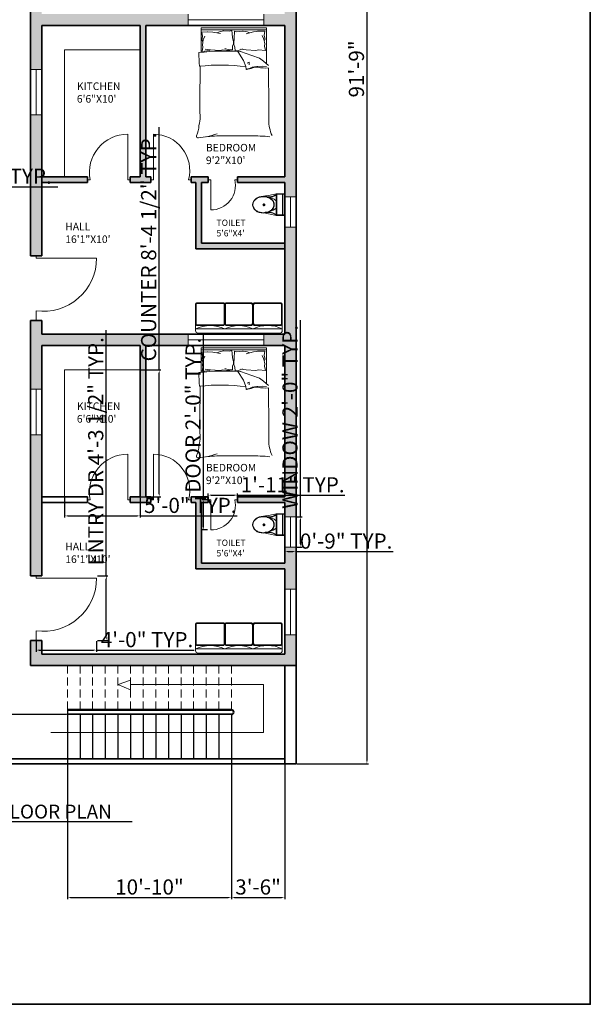
# Model space of a CAD drawing. Units: inches. Extents: x 1266 to 2869, y -408 to 3241.
# Tile 7 of 11: x 2416 to 2869, y 987 to 1767. Entities that reach past the tile are written whole.
import ezdxf

# ---------------------------------------------------------------- set-up
doc = ezdxf.new("R2010")
doc.units = ezdxf.units.IN
doc.linetypes.add('DASHED2', pattern=[9.525, 6.35, -3.175])
for name, color, linetype, lineweight in [('A-ANNO-DIMS', 2, 'Continuous', 18), ('A-ANNO-SYMB', 7, 'Continuous', 18), ('A-ANNO-TITL', 7, 'Continuous', 25), ('A-ANNO-TTLB', 7, 'Continuous', 35), ('A-AREA-IDEN', 7, 'Continuous', 18), ('A-DOOR', 4, 'Continuous', 18), ('A-FLOR-CASE', 9, 'Continuous', 18), ('A-FLOR-FIXT', 9, 'Continuous', 18), ('A-FLOR-STRS', 7, 'Continuous', 25), ('A-FLOR-STRS-OVHD', 8, 'DASHED2', 18), ('A-FURN', 8, 'Continuous', 18), ('A-GLAZ', 4, 'Continuous', 18), ('A-WALL', 7, 'Continuous', 35), ('A-WALL-PATT', 251, 'Continuous', 13)]:
    doc.layers.add(name, color=color, linetype=linetype, lineweight=lineweight)
doc.styles.get("Standard").update_dxf_attribs({"font": 'arial.ttf'})
doc.dimstyles.new('ISO-25', dxfattribs={"dimtxt": 12, "dimasz": 2.5, "dimexe": 1.25, "dimexo": 0.625, "dimtad": 1, "dimdec": 0, "dimlunit": 3, "dimtxsty": 'Standard', "dimcen": 2.5, "dimadec": 0, "dimazin": 0, "dimtfac": 1, "dimtdec": 0, "dimtmove": 0, "dimatfit": 3, "dimfxl": 1, "dimarcsym": 0})

# ---------------------------------------------------------------- blocks, each defined once
blk = doc.blocks.new('A$C31115884')
for p, q in [((283, 498), (223, 498)), ((258, 466), (258, 523)), ((0, 200), (0, 0)), ((520, 200), (0, 200)), ((510, 54), (0, 54)), ((10, 190), (10, 10)), ((510, 190), (10, 190)), ((10, 10), (510, 10)), ((510, 10), (510, 190)), ((520, 0), (520, 200)), ((0, 0), (520, 0))]:
    blk.add_line(p, q)
blk.add_circle((256, 496), 23.6)
for centre, radius, start, end in [((2778, -205), 2807, 165.4549, 171.7133), ((3237, 905), 2807, 188.2867, 194.5451), ((-295, 403), 365, 324.2091, 9.3499), ((-295, 403), 375, 324.2091, 9.3499), ((384, 406), 293, 190.2774, 224.1564), ((139, 406), 293, 315.8436, 2.6563), ((806, 403), 375, 179.2036, 215.7909), ((806, 403), 365, 170.6501, 215.7909)]:
    blk.add_arc(centre, radius, start, end)
blk.add_ellipse((256, 510), major_axis=(0, -261), ratio=0.772727)
blk.add_open_spline([(256, 259), (263, 259), (270, 260), (288, 262), (299, 265), (320, 273), (330, 278), (350, 291), (360, 299), (378, 316), (386, 326), (402, 347), (409, 358), (421, 383), (427, 395), (436, 422), (440, 436), (445, 465), (447, 480), (448, 509), (448, 524), (445, 553), (443, 568), (436, 596), (432, 610), (422, 636), (416, 649), (402, 672), (395, 683), (379, 703), (370, 712), (351, 728), (341, 735), (321, 746), (310, 751), (289, 757), (278, 759), (256, 761), (245, 761), (223, 757), (212, 754), (191, 746), (181, 741), (161, 728), (151, 720), (133, 703), (125, 693), (110, 672), (103, 660), (90, 636), (85, 623), (76, 596), (72, 582), (67, 553), (66, 538), (64, 509), (65, 494), (68, 465), (70, 450), (77, 422), (81, 408), (91, 382), (97, 370), (111, 346), (118, 335), (135, 316), (144, 307), (162, 291), (172, 284), (193, 273), (203, 269), (225, 262), (236, 260), (250, 259), (253, 259), (256, 259)], degree=3, knots=[0, 0, 0, 0, 0.110105, 0.110105, 0.285049, 0.285049, 0.459994, 0.459994, 0.634938, 0.634938, 0.809882, 0.809882, 0.984827, 0.984827, 1.159771, 1.159771, 1.334715, 1.334715, 1.50966, 1.50966, 1.684604, 1.684604, 1.859549, 1.859549, 2.034493, 2.034493, 2.209437, 2.209437, 2.384382, 2.384382, 2.559326, 2.559326, 2.73427, 2.73427, 2.909215, 2.909215, 3.084159, 3.084159, 3.259103, 3.259103, 3.434048, 3.434048, 3.608992, 3.608992, 3.783936, 3.783936, 3.958881, 3.958881, 4.133825, 4.133825, 4.30877, 4.30877, 4.483714, 4.483714, 4.658658, 4.658658, 4.833603, 4.833603, 5.008547, 5.008547, 5.183491, 5.183491, 5.358436, 5.358436, 5.53338, 5.53338, 5.708324, 5.708324, 5.883269, 5.883269, 6.058213, 6.058213, 6.233158, 6.233158, 6.283185, 6.283185, 6.283185, 6.283185])
blk = doc.blocks.new('*D5')
at = {"layer": 'A-ANNO-DIMS', "color": 0, "lineweight": -2, "transparency": 16777216}
for p, q in [((2636.08, 2278.35), (2692.86, 2278.35)), ((2691.61, 2275.85), (2691.61, 1179.85)), ((2636.08, 1177.35), (2692.86, 1177.35))]:
    blk.add_line(p, q, dxfattribs=at)
at = {"layer": 'A-ANNO-DIMS', "color": 0, "transparency": 16777216}
for points in [[(2691.19, 2275.85), (2692.02, 2275.85), (2691.61, 2278.35)], [(2691.19, 1179.85), (2692.02, 1179.85), (2691.61, 1177.35)]]:
    blk.add_solid(points, dxfattribs=at)
at = {"layer": 'Defpoints', "color": 0, "transparency": 16777216}
for p in [(2635.45, 2278.35), (2635.45, 1177.35), (2691.61, 1177.35)]:
    blk.add_point(p, dxfattribs=at)
at = {"layer": 'A-ANNO-DIMS', "color": 0, "transparency": 16777216, "insert": (2684.86, 1727.85), "char_height": 12, "attachment_point": 5, "rotation": 90}
blk.add_mtext('91\'-9"', dxfattribs=at)
blk = doc.blocks.new('BED-DOUBLE-2')
for p, q in [((3.76, 67.77), (3.76, 87.35)), ((3.76, 87.35), (55.42, 87.35)), ((55.42, 87.35), (55.42, 58.59)), ((3.76, 85.69), (55.42, 85.69)), ((4.21, 83.74), (8.84, 84.1)), ((4.21, 83.77), (4.84, 80.33)), ((4.84, 80.33), (4.37, 77.51)), ((5.46, 77.67), (6.55, 80.64)), ((8.84, 84.1), (8.96, 84.08)), ((8.96, 84.08), (13.09, 83.77)), ((13.09, 83.77), (19.03, 82.67)), ((16.06, 83.3), (18.25, 84.08)), ((18.25, 84.08), (21.37, 84.86)), ((21.37, 84.86), (21.72, 84.86)), ((21.72, 84.86), (26.53, 84.7)), ((26.53, 84.7), (28.09, 85.33)), ((28.09, 85.33), (28.71, 79.55)), ((28.71, 79.55), (29.34, 76.11)), ((29.98, 78.85), (29.57, 75.38)), ((30.24, 84.66), (29.98, 78.85)), ((31.84, 84.13), (30.24, 84.66)), ((36.63, 84.59), (31.84, 84.13)), ((36.98, 84.61), (36.63, 84.59)), ((40.14, 84.02), (36.98, 84.61)), ((45.31, 84.03), (39.45, 82.57)), ((42.38, 83.38), (40.14, 84.02)), ((49.42, 84.6), (45.31, 84.03)), ((54.17, 84.59), (48.33, 84.69)), ((48.33, 84.69), (49.42, 84.6)), ((53.31, 78.43), (52.03, 81.32)), ((54.17, 74.56), (53.31, 78.43)), ((54.17, 84.59), (53.76, 81.12)), ((53.76, 81.12), (54.41, 78.34)), ((54.41, 78.34), (53.85, 77.21)), ((4.37, 77.51), (4.99, 76.42)), ((4.52, 68.61), (5.15, 72.04)), ((4.84, 73.76), (5.46, 77.67)), ((5.15, 72.04), (4.84, 73.76)), ((6.9, 70.46), (11.26, 69.74)), ((26.06, 69.77), (22.66, 70.95)), ((29.34, 74.7), (28.71, 72.67)), ((28.71, 72.67), (28.71, 69.77)), ((29.34, 76.11), (29.34, 74.7)), ((29.57, 75.38), (29.66, 73.97)), ((29.66, 73.97), (30.41, 71.98)), ((30.41, 71.98), (30.59, 69.09)), ((33.24, 69.26), (36.56, 70.64)), ((35.2, 70.46), (39.56, 69.74)), ((53.97, 72.83), (54.17, 74.56)), ((54.81, 69.44), (53.97, 72.83)), ((10.03, 69.39), (4.52, 68.61)), ((11.26, 69.74), (10.03, 69.39)), ((11.26, 69.74), (18.84, 69.27)), ((18.84, 69.27), (20.95, 69.87)), ((20.95, 69.87), (26.5, 69.44)), ((28.71, 69.77), (26.06, 69.77)), ((30.59, 69.09), (33.24, 69.26)), ((32.71, 68.56), (37.24, 61.54)), ((43.94, 65.39), (34.92, 68.56)), ((39.56, 69.74), (47.14, 69.27)), ((49.96, 63.21), (43.94, 65.39)), ((47.14, 69.27), (49.26, 69.87)), ((49.26, 69.87), (54.81, 69.44)), ((53.15, 60.87), (49.96, 63.21)), ((37.24, 61.54), (39.08, 56.69)), ((39.08, 56.69), (39.42, 54.51)), ((39.42, 54.51), (42.1, 55.18)), ((40.12, 59.32), (41.78, 59.99)), ((41.87, 58.1), (41.78, 59.99, 4.18)), ((42.1, 55.18), (44.27, 56.19)), ((44.27, 56.19), (47.96, 56.69)), ((47.96, 56.69), (52.14, 57.02)), ((52.14, 57.02), (55.49, 56.69)), ((57.15, 57.36), (53.15, 60.87)), ((16.28, 1.69), (42.89, 1.69))]:
    blk.add_line(p, q)
for centre, radius, start, end in [((92.06, 65.63), 90.06, 178.72178, 185.60397), ((23.09, -109.45), 178.34, 86.08655, 96.78213), ((19.19, -81.63), 139.47, 81.78449, 96.90062), ((-180.86, 53.65), 183.89, 358.4762, 1.00819), ((33.68, 85.75), 32.06, 280.66171, 289.88058), ((47.29, 49.44), 6.73, 78.6608, 113.73842), ((55.49, 94.55), 39.11, 259.87628, 272.56571), ((197.03, 48.09), 139.99, 176.97912, 183.83645), ((524.11, 32.64), 521.39, 178.22771, 181.71854), ((39.61, 54.45), 0.199, 160.24637, 271.13765), ((-4874.07, 14.03), 4931.49, 0.00217, 0.28689), ((-29.08, 17.61), 32.04, 346.06484, 358.91125), ((-23.41, 11.38), 25.47, 337.97508, 356.652), ((82.33, 13.12), 24.93, 177.47136, 206.46809), ((1.18, 1.17), 1.18, 146.17358, 293.47814), ((23.16, -129.76), 131.62, 92.99578, 99.40907), ((-18.62, 112.98), 115.08, 283.38322, 287.70533), ((44.49, -142.12), 143.82, 84.4998, 90.63509)]:
    blk.add_arc(centre, radius, start, end)
blk = doc.blocks.new('DOOR-KITCHEN-R')
for p, q in [((31.78, 0), (31.78, 36)), ((0, 0), (2, 0)), ((33.78, 0), (31.78, 0))]:
    blk.add_line(p, q)
blk.add_arc((31.78, 5.68), 30.32, 90, 190.7956)
blk = doc.blocks.new('DOOR-BEDROOM-R')
for p, q in [((2, 0), (2, 36)), ((0, 0), (2, 0)), ((31.84, 0), (29.84, 0))]:
    blk.add_line(p, q)
blk.add_arc((2, 7.24), 28.76, 345.43182, 90)
blk = doc.blocks.new('DOOR-BATH-R')
for p, q in [((0, 24), (2, 24)), ((2, 24), (2, 0)), ((23.14, 24), (21.14, 24))]:
    blk.add_line(p, q)
blk.add_arc((2, 19.63), 19.63, 270, 12.84994)
blk = doc.blocks.new('DOOR-ENTRY-R')
for p, q in [((0, 51.27), (0, 49.27)), ((0, 49.27), (36, 49.27)), ((36, 49.27), (48, 49.27)), ((0, 5.68), (0, 7.68)), ((0, 0), (0, 5.68))]:
    blk.add_line(p, q)
blk.add_arc((5.98, 49.27), 42.02, 261.81164, 0)
blk = doc.blocks.new('WIN-PLAN-60')
for p, q in [((0, 9), (0, 0)), ((60, 4.5), (60, 9)), ((60, 9), (60, 0)), ((0, 4.5), (60, 4.5)), ((0, 0), (0, 4.5))]:
    blk.add_line(p, q)
blk = doc.blocks.new('WIN-PLAN-36')
for p, q in [((0, 36), (9, 36)), ((4.5, 36), (4.5, 0)), ((9, 36), (4.5, 36)), ((4.5, 0), (0, 0)), ((0, 0), (9, 0))]:
    blk.add_line(p, q)
blk = doc.blocks.new('WIN-PLAN-24')
for p, q in [((0, 24), (9, 24)), ((4.5, 24), (4.5, 0)), ((9, 24), (4.5, 24)), ((0, 0), (9, 0))]:
    blk.add_line(p, q)
blk = doc.blocks.new('COUNTER-KITCHEN')
for p, q in [((0, 0), (0, 100.54)), ((0, 100.54), (59.82, 100.54))]:
    blk.add_line(p, q)
blk = doc.blocks.new('STAIR-PATH-RETURN')
for p, q in [((63.2, 41.3), (53.5, 38.03)), ((63.2, 33.87), (63.2, 41.3)), ((53.2, 38.03), (63.2, 33.87)), ((53.5, 38.03), (53.2, 38.03)), ((168.66, 38.03), (63.2, 38.03)), ((168.66, 0), (168.66, 38.03)), ((0, 0), (168.66, 0))]:
    blk.add_line(p, q)
blk = doc.blocks.new('*D43')
at = {"layer": 'A-ANNO-DIMS', "color": 0, "lineweight": -2, "transparency": 16777216}
for p, q in [((2197.56, 1639.47), (2197.56, 1633.21)), ((2235.18, 1639.47), (2235.18, 1633.21)), ((2200.06, 1634.46), (2232.68, 1634.46)), ((2235.18, 1634.46), (2446.61, 1634.46))]:
    blk.add_line(p, q, dxfattribs=at)
at = {"layer": 'A-ANNO-DIMS', "color": 0, "transparency": 16777216}
for points in [[(2200.06, 1634.87), (2200.06, 1634.04), (2197.56, 1634.46)], [(2232.68, 1634.87), (2232.68, 1634.04), (2235.18, 1634.46)]]:
    blk.add_solid(points, dxfattribs=at)
at = {"layer": 'Defpoints', "color": 0, "transparency": 16777216}
for p in [(2197.56, 1640.1), (2235.18, 1640.1), (2235.18, 1634.46)]:
    blk.add_point(p, dxfattribs=at)
at = {"layer": 'A-ANNO-DIMS', "color": 0, "transparency": 16777216, "insert": (2342.14, 1641.29), "char_height": 12, "attachment_point": 5}
blk.add_mtext('KITCHEN DR 3\'-1 1/2" TYP.', dxfattribs=at)
blk = doc.blocks.new('*D49')
at = {"layer": 'A-ANNO-DIMS', "color": 0, "lineweight": -2, "transparency": 16777216}
for p, q in [((2527.03, 1489.38), (2527.03, 1681.65)), ((2512.58, 1489.38), (2528.28, 1489.38)), ((2527.03, 1391.35), (2527.03, 1486.88)), ((2512.58, 1388.85), (2528.28, 1388.85))]:
    blk.add_line(p, q, dxfattribs=at)
at = {"layer": 'A-ANNO-DIMS', "color": 0, "transparency": 16777216}
for points in [[(2526.61, 1486.88), (2527.45, 1486.88), (2527.03, 1489.38)], [(2526.61, 1391.35), (2527.45, 1391.35), (2527.03, 1388.85)]]:
    blk.add_solid(points, dxfattribs=at)
at = {"layer": 'Defpoints', "color": 0, "transparency": 16777216}
for p in [(2511.95, 1489.38), (2527.03, 1489.38), (2511.95, 1388.85)]:
    blk.add_point(p, dxfattribs=at)
at = {"layer": 'A-ANNO-DIMS', "color": 0, "transparency": 16777216, "insert": (2520.2, 1586.77), "char_height": 12, "attachment_point": 5, "rotation": 90}
blk.add_mtext('COUNTER 8\'-4 1/2" TYP.', dxfattribs=at)
blk = doc.blocks.new('*D50')
at = {"layer": 'A-ANNO-DIMS', "color": 0, "lineweight": -2, "transparency": 16777216}
for p, q in [((2452.13, 1388.22), (2452.13, 1372.52)), ((2511.95, 1388.22), (2511.95, 1372.52)), ((2454.63, 1373.77), (2509.45, 1373.77)), ((2511.95, 1373.77), (2588.85, 1373.77))]:
    blk.add_line(p, q, dxfattribs=at)
at = {"layer": 'A-ANNO-DIMS', "color": 0, "transparency": 16777216}
for points in [[(2454.63, 1374.18), (2454.63, 1373.35), (2452.13, 1373.77)], [(2509.45, 1374.18), (2509.45, 1373.35), (2511.95, 1373.77)]]:
    blk.add_solid(points, dxfattribs=at)
at = {"layer": 'Defpoints', "color": 0, "transparency": 16777216}
for p in [(2452.13, 1388.85), (2511.95, 1388.85), (2511.95, 1373.77)]:
    blk.add_point(p, dxfattribs=at)
at = {"layer": 'A-ANNO-DIMS', "color": 0, "transparency": 16777216, "insert": (2551.65, 1380.52), "char_height": 12, "attachment_point": 5}
blk.add_mtext('5\'-0" TYP.', dxfattribs=at)
blk = doc.blocks.new('*D57')
at = {"layer": 'A-ANNO-DIMS', "color": 0, "lineweight": -2, "transparency": 16777216}
for p, q in [((2562.24, 1386.6), (2562.24, 1517.85)), ((2565.21, 1386.6), (2560.99, 1386.6)), ((2562.24, 1365.1), (2562.24, 1384.1)), ((2565.21, 1362.6), (2560.99, 1362.6))]:
    blk.add_line(p, q, dxfattribs=at)
at = {"layer": 'A-ANNO-DIMS', "color": 0, "transparency": 16777216}
for points in [[(2561.82, 1384.1), (2562.65, 1384.1), (2562.24, 1386.6)], [(2561.82, 1365.1), (2562.65, 1365.1), (2562.24, 1362.6)]]:
    blk.add_solid(points, dxfattribs=at)
at = {"layer": 'Defpoints', "color": 0, "transparency": 16777216}
for p in [(2562.24, 1386.6), (2565.84, 1386.6), (2565.84, 1362.6)]:
    blk.add_point(p, dxfattribs=at)
at = {"layer": 'A-ANNO-DIMS', "color": 0, "transparency": 16777216, "insert": (2555.4, 1453.47), "char_height": 12, "attachment_point": 5, "rotation": 90}
blk.add_mtext('DOOR 2\'-0" TYP.', dxfattribs=at)
blk = doc.blocks.new('*D58')
at = {"layer": 'A-ANNO-DIMS', "color": 0, "lineweight": -2, "transparency": 16777216}
for p, q in [((2565.84, 1387.22), (2565.84, 1391.45)), ((2568.34, 1390.2), (2586.48, 1390.2)), ((2588.98, 1387.22), (2588.98, 1391.45)), ((2588.98, 1390.2), (2674.07, 1390.2))]:
    blk.add_line(p, q, dxfattribs=at)
at = {"layer": 'A-ANNO-DIMS', "color": 0, "transparency": 16777216}
for points in [[(2568.34, 1390.61), (2568.34, 1389.78), (2565.84, 1390.2)], [(2586.48, 1390.61), (2586.48, 1389.78), (2588.98, 1390.2)]]:
    blk.add_solid(points, dxfattribs=at)
at = {"layer": 'Defpoints', "color": 0, "transparency": 16777216}
for p in [(2588.98, 1390.2), (2565.84, 1386.6), (2588.98, 1386.6)]:
    blk.add_point(p, dxfattribs=at)
at = {"layer": 'A-ANNO-DIMS', "color": 0, "transparency": 16777216, "insert": (2632.77, 1396.85), "char_height": 12, "attachment_point": 5}
blk.add_mtext('1\'-11" TYP.', dxfattribs=at)
blk = doc.blocks.new('*D59')
at = {"layer": 'A-ANNO-DIMS', "color": 0, "lineweight": -2, "transparency": 16777216}
for p, q in [((2485.14, 1326.39), (2485.14, 1520.96)), ((2478.08, 1326.39), (2486.39, 1326.39)), ((2485.14, 1277.62), (2485.14, 1323.89)), ((2478.08, 1275.12), (2486.39, 1275.12))]:
    blk.add_line(p, q, dxfattribs=at)
at = {"layer": 'A-ANNO-DIMS', "color": 0, "transparency": 16777216}
for points in [[(2484.72, 1323.89), (2485.56, 1323.89), (2485.14, 1326.39)], [(2484.72, 1277.62), (2485.56, 1277.62), (2485.14, 1275.12)]]:
    blk.add_solid(points, dxfattribs=at)
at = {"layer": 'Defpoints', "color": 0, "transparency": 16777216}
for p in [(2477.45, 1326.39), (2485.14, 1326.39), (2477.45, 1275.12)]:
    blk.add_point(p, dxfattribs=at)
at = {"layer": 'A-ANNO-DIMS', "color": 0, "transparency": 16777216, "insert": (2478.31, 1424.92), "char_height": 12, "attachment_point": 5, "rotation": 90}
blk.add_mtext('ENTRY DR 4\'-3 1/2" TYP.', dxfattribs=at)
blk = doc.blocks.new('*D60')
at = {"layer": 'A-ANNO-DIMS', "color": 0, "lineweight": -2, "transparency": 16777216}
for p, q in [((2429.45, 1274.49), (2429.45, 1266.18)), ((2477.45, 1274.49), (2477.45, 1266.18)), ((2431.95, 1267.43), (2474.95, 1267.43)), ((2477.45, 1267.43), (2554.83, 1267.43))]:
    blk.add_line(p, q, dxfattribs=at)
at = {"layer": 'A-ANNO-DIMS', "color": 0, "transparency": 16777216}
for points in [[(2431.95, 1267.84), (2431.95, 1267.01), (2429.45, 1267.43)], [(2474.95, 1267.84), (2474.95, 1267.01), (2477.45, 1267.43)]]:
    blk.add_solid(points, dxfattribs=at)
at = {"layer": 'Defpoints', "color": 0, "transparency": 16777216}
for p in [(2429.45, 1275.12), (2477.45, 1275.12), (2477.45, 1267.43)]:
    blk.add_point(p, dxfattribs=at)
at = {"layer": 'A-ANNO-DIMS', "color": 0, "transparency": 16777216, "insert": (2517.39, 1274.18), "char_height": 12, "attachment_point": 5}
blk.add_mtext('4\'-0" TYP.', dxfattribs=at)
blk = doc.blocks.new('*D61')
at = {"layer": 'A-ANNO-DIMS', "color": 0, "lineweight": -2, "transparency": 16777216}
for p, q in [((2639.05, 1373.11), (2639.05, 1528.71)), ((2636.08, 1373.11), (2640.3, 1373.11)), ((2639.05, 1351.61), (2639.05, 1370.61)), ((2636.08, 1349.11), (2640.3, 1349.11))]:
    blk.add_line(p, q, dxfattribs=at)
at = {"layer": 'A-ANNO-DIMS', "color": 0, "transparency": 16777216}
for points in [[(2638.63, 1370.61), (2639.47, 1370.61), (2639.05, 1373.11)], [(2638.63, 1351.61), (2639.47, 1351.61), (2639.05, 1349.11)]]:
    blk.add_solid(points, dxfattribs=at)
at = {"layer": 'Defpoints', "color": 0, "transparency": 16777216}
for p in [(2635.45, 1373.11), (2639.05, 1373.11), (2635.45, 1349.11)]:
    blk.add_point(p, dxfattribs=at)
at = {"layer": 'A-ANNO-DIMS', "color": 0, "transparency": 16777216, "insert": (2632.22, 1452.16), "char_height": 12, "attachment_point": 5, "rotation": 90}
blk.add_mtext('WINDOW 2\'-0" TYP.', dxfattribs=at)
blk = doc.blocks.new('*D62')
at = {"layer": 'A-ANNO-DIMS', "color": 0, "lineweight": -2, "transparency": 16777216}
for p, q in [((2626.45, 1348.48), (2626.45, 1344.26)), ((2628.95, 1345.51), (2632.95, 1345.51)), ((2635.45, 1348.48), (2635.45, 1344.26)), ((2635.45, 1345.51), (2712.35, 1345.51))]:
    blk.add_line(p, q, dxfattribs=at)
at = {"layer": 'A-ANNO-DIMS', "color": 0, "transparency": 16777216}
for points in [[(2628.95, 1345.93), (2628.95, 1345.09), (2626.45, 1345.51)], [(2632.95, 1345.93), (2632.95, 1345.09), (2635.45, 1345.51)]]:
    blk.add_solid(points, dxfattribs=at)
at = {"layer": 'Defpoints', "color": 0, "transparency": 16777216}
for p in [(2626.45, 1349.11), (2635.45, 1349.11), (2635.45, 1345.51)]:
    blk.add_point(p, dxfattribs=at)
at = {"layer": 'A-ANNO-DIMS', "color": 0, "transparency": 16777216, "insert": (2675.15, 1352.26), "char_height": 12, "attachment_point": 5}
blk.add_mtext('0\'-9" TYP.', dxfattribs=at)
blk = doc.blocks.new('*D85')
at = {"layer": 'A-ANNO-DIMS', "color": 0, "lineweight": -2, "transparency": 16777216}
for p, q in [((2454.31, 1180.78), (2454.31, 1070.23)), ((2584.31, 1180.78), (2584.31, 1070.23)), ((2456.81, 1071.48), (2581.81, 1071.48))]:
    blk.add_line(p, q, dxfattribs=at)
at = {"layer": 'A-ANNO-DIMS', "color": 0, "transparency": 16777216}
for points in [[(2456.81, 1071.9), (2456.81, 1071.06), (2454.31, 1071.48)], [(2581.81, 1071.9), (2581.81, 1071.06), (2584.31, 1071.48)]]:
    blk.add_solid(points, dxfattribs=at)
at = {"layer": 'Defpoints', "color": 0, "transparency": 16777216}
for p in [(2454.31, 1181.4), (2584.31, 1181.4), (2584.31, 1071.48)]:
    blk.add_point(p, dxfattribs=at)
at = {"layer": 'A-ANNO-DIMS', "color": 0, "transparency": 16777216, "insert": (2519.31, 1078.23), "char_height": 12, "attachment_point": 5}
blk.add_mtext('10\'-10"', dxfattribs=at)
blk = doc.blocks.new('*D86')
at = {"layer": 'A-ANNO-DIMS', "color": 0, "lineweight": -2, "transparency": 16777216}
for p, q in [((2584.31, 1180.78), (2584.31, 1070.23)), ((2626.45, 1180.78), (2626.45, 1070.23)), ((2586.81, 1071.48), (2623.95, 1071.48))]:
    blk.add_line(p, q, dxfattribs=at)
at = {"layer": 'A-ANNO-DIMS', "color": 0, "transparency": 16777216}
for points in [[(2586.81, 1071.9), (2586.81, 1071.06), (2584.31, 1071.48)], [(2623.95, 1071.9), (2623.95, 1071.06), (2626.45, 1071.48)]]:
    blk.add_solid(points, dxfattribs=at)
at = {"layer": 'Defpoints', "color": 0, "transparency": 16777216}
for p in [(2584.31, 1181.4), (2626.45, 1181.4), (2626.45, 1071.48)]:
    blk.add_point(p, dxfattribs=at)
at = {"layer": 'A-ANNO-DIMS', "color": 0, "transparency": 16777216, "insert": (2605.38, 1078.23), "char_height": 12, "attachment_point": 5}
blk.add_mtext('3\'-6"', dxfattribs=at)
blk = doc.blocks.new('*D87')
at = {"layer": 'A-ANNO-DIMS', "color": 0, "lineweight": -2, "transparency": 16777216}
for p, q in [((1969.26, 1216.35), (1969.26, 1261.52)), ((2453.69, 1216.35), (1968.01, 1216.35)), ((1969.26, 1183.9), (1969.26, 1213.85)), ((2453.69, 1181.4), (1968.01, 1181.4))]:
    blk.add_line(p, q, dxfattribs=at)
at = {"layer": 'A-ANNO-DIMS', "color": 0, "transparency": 16777216}
for points in [[(1968.84, 1213.85), (1969.68, 1213.85), (1969.26, 1216.35)], [(1968.84, 1183.9), (1969.68, 1183.9), (1969.26, 1181.4)]]:
    blk.add_solid(points, dxfattribs=at)
at = {"layer": 'Defpoints', "color": 0, "transparency": 16777216}
for p in [(1969.26, 1216.35), (2454.31, 1216.35), (2454.31, 1181.4)]:
    blk.add_point(p, dxfattribs=at)
at = {"layer": 'A-ANNO-DIMS', "color": 0, "transparency": 16777216, "insert": (1962.61, 1240.19), "char_height": 12, "attachment_point": 5, "rotation": 90}
blk.add_mtext('2\'-11"', dxfattribs=at)

msp = doc.modelspace()

# ---------------------------------------------------------------- hatches: boundary and pattern name
at = {"layer": 'A-WALL-PATT'}
h = msp.add_hatch(color=256, dxfattribs=at)
h.dxf.hatch_style = 1
h.paths.add_polyline_path([(2161.45, 2269.35), (2239.45, 2269.35), (2239.45, 2149.35), (2235.18, 2149.35), (2235.18, 2144.85), (2243.95, 2144.85), (2249.99, 2144.85), (2249.99, 2146.74), (2249.99, 2149.35), (2243.95, 2149.35), (2243.95, 2269.35), (2274.21, 2269.35), (2274.21, 2273.85), (2274.21, 2278.35), (2152.45, 2278.35), (2152.45, 2234.52), (2161.45, 2234.52)])
h.paths.add_polyline_path([(2550.01, 2278.35), (2424.95, 2278.35), (2372.95, 2278.35), (2334.21, 2278.35), (2334.21, 2269.35), (2363.95, 2269.35), (2363.95, 2149.35), (2328.7, 2149.35), (2328.7, 2144.85), (2363.95, 2144.85), (2363.95, 2133.61), (2372.95, 2133.61), (2372.95, 2269.35), (2424.95, 2269.35), (2424.95, 2234.52), (2433.95, 2234.52), (2433.95, 2269.35), (2511.95, 2269.35), (2511.95, 2149.35), (2504.09, 2149.35), (2504.09, 2144.85), (2520.49, 2144.85), (2520.49, 2149.35), (2516.45, 2149.35), (2516.45, 2269.35), (2550.01, 2269.35), (2550.01, 2273.85)])
h.paths.add_polyline_path([(2635.45, 2278.35), (2610.01, 2278.35), (2610.01, 2269.35), (2626.45, 2269.35), (2626.45, 2149.35), (2588.98, 2149.35), (2588.98, 2144.85), (2626.45, 2144.85), (2626.45, 2133.61), (2635.45, 2133.61)])
h.paths.add_polyline_path([(2560.45, 2144.85), (2565.84, 2144.85), (2565.84, 2149.35), (2552.33, 2149.35), (2552.33, 2144.85), (2555.95, 2144.85), (2555.95, 2092.35), (2626.45, 2092.35), (2626.45, 2086.89), (2626.45, 2024.85), (2610.01, 2024.85), (2610.01, 2015.85), (2626.45, 2015.85), (2626.45, 1895.85), (2589.21, 1895.85), (2589.21, 1891.35), (2626.45, 1891.35), (2626.45, 1880.11), (2635.45, 1880.11), (2635.45, 2086.89), (2635.45, 2109.61), (2626.45, 2109.61), (2626.45, 2096.85), (2560.45, 2096.85)])
h.paths.add_polyline_path([(2433.95, 2198.52), (2424.95, 2198.52), (2424.95, 2086.89), (2433.95, 2086.89), (2433.95, 2144.85), (2470.3, 2144.85), (2470.3, 2149.35), (2433.95, 2149.35)])
h.paths.add_polyline_path([(2372.95, 2109.61), (2363.95, 2109.61), (2363.95, 2096.85), (2297.95, 2096.85), (2297.95, 2144.85), (2304, 2144.85), (2304, 2149.35), (2293.45, 2149.35), (2287.11, 2149.35), (2287.11, 2144.85), (2293.45, 2144.85), (2293.45, 2092.35), (2363.95, 2092.35), (2363.95, 2086.89), (2372.95, 2086.89)], flags=17)
h.paths.add_polyline_path([(2161.45, 2144.85), (2197.56, 2144.85), (2197.56, 2149.35), (2161.45, 2149.35), (2161.45, 2198.52), (2152.45, 2198.52), (2152.45, 1981.02), (2161.45, 1981.02), (2161.45, 2015.85), (2363.95, 2015.85), (2363.95, 1895.85), (2326.89, 1895.85), (2326.89, 1891.35), (2363.95, 1891.35), (2363.95, 1880.11), (2372.95, 1880.11), (2372.95, 2035.62), (2363.95, 2035.62), (2363.95, 2024.85), (2161.45, 2024.85)])
h.paths.add_polyline_path([(2161.45, 1691.52), (2152.45, 1691.52), (2152.45, 1474.02), (2161.45, 1474.02)])
h.paths.add_polyline_path([(2194.79, 1895.85), (2161.45, 1895.85), (2161.45, 1945.02), (2152.45, 1945.02), (2152.45, 1727.52), (2161.45, 1727.52), (2161.45, 1762.35), (2363.95, 1762.35), (2363.95, 1642.35), (2328.7, 1642.35), (2328.7, 1637.85), (2363.95, 1637.85), (2363.95, 1589.85), (2297.95, 1589.85), (2297.95, 1637.85), (2303.95, 1637.85), (2303.95, 1642.35), (2287.64, 1642.35), (2287.64, 1637.85), (2293.45, 1637.85), (2293.45, 1585.35), (2363.95, 1585.35), (2363.95, 1579.45), (2372.95, 1579.45), (2372.95, 1779.84), (2363.95, 1779.84), (2363.95, 1771.35), (2161.45, 1771.35), (2161.45, 1891.35), (2194.79, 1891.35)])
h.paths.add_polyline_path([(2243.95, 2015.85), (2239.45, 2015.85), (2239.45, 1895.85), (2232.4, 1895.85), (2232.4, 1891.35), (2247.22, 1891.35), (2247.22, 1895.85), (2243.95, 1895.85)], flags=17)
h.paths.add_polyline_path([(2302.19, 1895.85), (2284.34, 1895.85), (2284.34, 1891.35), (2293.45, 1891.35), (2293.45, 1838.85), (2363.95, 1838.85), (2363.95, 1831.11), (2372.95, 1831.11), (2372.95, 1856.11), (2363.95, 1856.11), (2363.95, 1843.35), (2297.95, 1843.35), (2297.95, 1891.35), (2302.19, 1891.35)], flags=17)
h.paths.add_polyline_path([(2243.95, 1762.35), (2239.45, 1762.35), (2239.45, 1642.35), (2235.18, 1642.35), (2235.18, 1637.85), (2249.99, 1637.85), (2249.99, 1642.35), (2243.95, 1642.35)], flags=17)
h.paths.add_polyline_path([(2197.56, 1642.35), (2161.45, 1642.35), (2161.45, 1637.85), (2197.56, 1637.85)], flags=17)
h.paths.add_polyline_path([(2363.95, 1517.85), (2161.45, 1517.85), (2161.45, 1508.85), (2239.45, 1508.85), (2239.45, 1388.85), (2243.95, 1388.85), (2243.95, 1508.85), (2363.95, 1508.85)])
h.paths.add_polyline_path([(2372.95, 1528.18), (2363.95, 1528.18), (2363.95, 1323.21), (2372.95, 1323.21)])
h.paths.add_polyline_path([(2372.95, 1271.94), (2363.95, 1271.94), (2363.95, 1264.35), (2161.45, 1264.35), (2161.45, 1283.77), (2156.95, 1283.77), (2152.45, 1283.77), (2152.45, 1255.35), (2156.95, 1255.35), (2372.95, 1255.35)])
h.paths.add_polyline_path([(2161.45, 1438.02), (2152.45, 1438.02), (2152.45, 1319.77), (2161.45, 1319.77)])
h.paths.add_polyline_path([(2550.01, 1513.35), (2550.01, 1517.85), (2433.95, 1517.85), (2433.95, 1528.62), (2424.95, 1528.62), (2424.95, 1474.02), (2433.95, 1474.02), (2433.95, 1508.85), (2511.95, 1508.85), (2511.95, 1388.85), (2504.09, 1388.85), (2504.09, 1384.35), (2520.49, 1384.35), (2520.49, 1388.85), (2516.45, 1388.85), (2516.45, 1508.85), (2550.01, 1508.85)])
h.paths.add_polyline_path([(2635.45, 1602.61), (2626.45, 1602.61), (2626.45, 1517.85), (2610.01, 1517.85), (2610.01, 1508.85), (2626.45, 1508.85), (2626.45, 1388.85), (2588.98, 1388.85), (2588.98, 1384.35), (2626.45, 1384.35), (2626.45, 1373.11), (2635.45, 1373.11)])
h.paths.add_polyline_path([(2635.45, 1349.11), (2626.45, 1349.11), (2626.45, 1336.35), (2560.45, 1336.35), (2560.45, 1384.35), (2565.84, 1384.35), (2565.84, 1388.85), (2552.33, 1388.85), (2552.33, 1384.35), (2555.95, 1384.35), (2555.95, 1331.85), (2626.45, 1331.85), (2626.45, 1315.59), (2635.45, 1315.59)])
h.paths.add_polyline_path([(2635.45, 1279.59), (2630.95, 1279.59), (2626.45, 1279.59), (2626.45, 1264.35), (2433.95, 1264.35), (2433.95, 1275.12), (2424.95, 1275.12), (2424.95, 1255.35), (2635.45, 1255.35)])
h.paths.add_polyline_path([(2433.95, 1438.02), (2424.95, 1438.02), (2424.95, 1326.39), (2433.95, 1326.39)])
h.paths.add_polyline_path([(2470.3, 1388.85), (2433.95, 1388.85), (2433.95, 1384.35), (2470.3, 1384.35)], flags=0)
h = msp.add_hatch(color=256, dxfattribs=at)
h.dxf.hatch_style = 1
h.paths.add_polyline_path([(2550.01, 2020.35), (2550.01, 2024.85), (2433.95, 2024.85), (2433.95, 2035.62), (2424.95, 2035.62), (2424.95, 1981.02), (2433.95, 1981.02), (2433.95, 2015.85), (2511.95, 2015.85), (2511.95, 1895.85), (2504.33, 1895.85), (2504.33, 1891.35), (2520.72, 1891.35), (2520.72, 1895.85), (2516.45, 1895.85), (2516.45, 2015.85), (2550.01, 2015.85)])
h.paths.add_polyline_path([(2433.95, 1945.02), (2424.95, 1945.02), (2424.95, 1833.39), (2433.95, 1833.39), (2433.95, 1891.35), (2470.53, 1891.35), (2470.53, 1895.85), (2433.95, 1895.85)])
h.paths.add_polyline_path([(2550.01, 1771.35), (2433.95, 1771.35), (2433.95, 1787.8), (2424.95, 1787.8), (2424.95, 1727.52), (2433.95, 1727.52), (2433.95, 1762.35), (2511.95, 1762.35), (2511.95, 1642.35), (2504.09, 1642.35), (2504.09, 1637.85), (2520.49, 1637.85), (2520.49, 1642.35), (2516.45, 1642.35), (2516.45, 1762.35), (2550.01, 1762.35), (2550.01, 1766.85)])
h.paths.add_polyline_path([(2560.45, 1637.85), (2565.84, 1637.85), (2565.84, 1642.35), (2552.33, 1642.35), (2552.33, 1637.85), (2555.95, 1637.85), (2555.95, 1585.35), (2626.45, 1585.35), (2626.45, 1589.85), (2560.45, 1589.85)])
h.paths.add_polyline_path([(2635.45, 1856.11), (2626.45, 1856.11), (2626.45, 1843.35), (2560.45, 1843.35), (2560.45, 1891.35), (2566.07, 1891.35), (2566.07, 1895.85), (2552.56, 1895.85), (2552.56, 1891.35), (2555.95, 1891.35), (2555.95, 1838.85), (2626.45, 1838.85), (2626.45, 1771.35), (2610.01, 1771.35), (2610.01, 1762.35), (2626.45, 1762.35), (2626.45, 1642.35), (2588.98, 1642.35), (2588.98, 1637.85), (2626.45, 1637.85), (2626.45, 1626.61), (2635.45, 1626.61)])
h.paths.add_polyline_path([(2433.95, 1691.52), (2424.95, 1691.52), (2424.95, 1579.89), (2433.95, 1579.89)])
h.paths.add_polyline_path([(2470.3, 1642.35), (2433.95, 1642.35), (2433.95, 1637.85), (2470.3, 1637.85)], flags=17)

# ---------------------------------------------------------------- linework, layer by layer
at = {"layer": 'A-ANNO-TITL'}
msp.add_line((2333.33, 1131.68), (2505.49, 1131.68), dxfattribs=at)
at = {"layer": 'A-ANNO-TTLB'}
msp.add_lwpolyline([(1266.23, 3241.34), (2868.62, 3241.34), (2868.62, 986.84), (1266.23, 986.84)], close=True, dxfattribs=at)
at = {"layer": 'A-FLOR-STRS'}
for p, q in [((2584.31, 1220.35), (2454.31, 1220.35)), ((2454.31, 1220.35), (2454.31, 1216.35)), ((2454.31, 1220.35), (2454.31, 1219.85)), ((2454.31, 1219.85), (2584.31, 1219.85)), ((2454.31, 1216.35), (2454.31, 1216.85)), ((2454.31, 1216.85), (2584.31, 1216.85)), ((2584.31, 1216.35), (2454.31, 1216.35)), ((2454.31, 1216.35), (2454.31, 1181.4)), ((2464.31, 1216.35), (2464.31, 1181.4)), ((2474.31, 1216.35), (2474.31, 1181.4)), ((2484.31, 1216.35), (2484.31, 1181.4)), ((2494.31, 1216.35), (2494.31, 1181.4)), ((2504.31, 1216.35), (2504.31, 1181.4)), ((2514.31, 1216.35), (2514.31, 1181.4)), ((2524.31, 1216.35), (2524.31, 1181.4)), ((2534.31, 1216.35), (2534.31, 1181.4)), ((2544.31, 1216.35), (2544.31, 1181.4)), ((2554.31, 1216.35), (2554.31, 1181.4)), ((2564.31, 1216.35), (2564.31, 1181.4)), ((2574.31, 1216.35), (2574.31, 1181.4)), ((2584.31, 1216.35), (2584.31, 1181.4))]:
    msp.add_line(p, q, dxfattribs=at)
for radius in [2, 1.5]:
    msp.add_arc((2584.31, 1218.35), radius, 270, 90, dxfattribs=at)
at = {"layer": 'A-FLOR-STRS-OVHD'}
for p, q in [((2454.31, 1220.35), (2454.31, 1255.35)), ((2464.31, 1220.35), (2464.31, 1255.35)), ((2474.31, 1220.35), (2474.31, 1255.35)), ((2484.31, 1220.35), (2484.31, 1255.35)), ((2494.31, 1220.35), (2494.31, 1255.35)), ((2504.31, 1220.35), (2504.31, 1255.35)), ((2514.31, 1220.35), (2514.31, 1255.35)), ((2524.31, 1220.35), (2524.31, 1255.35)), ((2534.31, 1220.35), (2534.31, 1255.35)), ((2544.31, 1220.35), (2544.31, 1255.35)), ((2554.31, 1220.35), (2554.31, 1255.35)), ((2564.31, 1220.35), (2564.31, 1255.35)), ((2574.31, 1220.35), (2574.31, 1255.35)), ((2584.31, 1220.35), (2584.31, 1255.35))]:
    msp.add_line(p, q, dxfattribs=at)
at = {"layer": 'A-FURN'}
for points in [[(2555.77, 1540.88), (2555.77, 1526.26, 0.414214), (2557.49, 1524.54), (2577.27, 1524.54, 0.414214), (2578.99, 1526.26), (2578.99, 1540.88, 0.414214), (2577.27, 1542.6), (2557.49, 1542.6, 0.414214)], [(2556.29, 1540.88), (2556.29, 1526.26, 0.414214), (2557.49, 1525.06), (2577.27, 1525.06, 0.414214), (2578.48, 1526.26), (2578.48, 1540.88, 0.414214), (2577.27, 1542.09), (2557.49, 1542.09, 0.414214)], [(2601.35, 1540.88), (2601.35, 1526.26, -0.414214), (2599.63, 1524.54), (2580.71, 1524.54, -0.414214), (2578.99, 1526.26), (2578.99, 1540.88, -0.414214), (2580.71, 1542.6), (2599.63, 1542.6, -0.414214)], [(2600.83, 1540.88), (2600.83, 1526.26, -0.414214), (2599.63, 1525.06), (2580.71, 1525.06, -0.414214), (2579.51, 1526.26), (2579.51, 1540.88, -0.414214), (2580.71, 1542.09), (2599.63, 1542.09, -0.414214)], [(2601.35, 1540.88), (2601.35, 1526.26, 0.414214), (2603.07, 1524.54), (2622.85, 1524.54, 0.414214), (2624.57, 1526.26), (2624.57, 1540.88, 0.414214), (2622.85, 1542.6), (2603.07, 1542.6, 0.414214)], [(2601.86, 1540.88), (2601.86, 1526.26, 0.414214), (2603.07, 1525.06), (2622.85, 1525.06, 0.414214), (2624.05, 1526.26), (2624.05, 1540.88, 0.414214), (2622.85, 1542.09), (2603.07, 1542.09, 0.414214)], [(2555.77, 1287.38), (2555.77, 1272.76, 0.414214), (2557.49, 1271.04), (2577.27, 1271.04, 0.414214), (2578.99, 1272.76), (2578.99, 1287.38, 0.414214), (2577.27, 1289.1), (2557.49, 1289.1, 0.414214)], [(2556.29, 1287.38), (2556.29, 1272.76, 0.414214), (2557.49, 1271.56), (2577.27, 1271.56, 0.414214), (2578.48, 1272.76), (2578.48, 1287.38, 0.414214), (2577.27, 1288.59), (2557.49, 1288.59, 0.414214)], [(2601.35, 1287.38), (2601.35, 1272.76, -0.414214), (2599.63, 1271.04), (2580.71, 1271.04, -0.414214), (2578.99, 1272.76), (2578.99, 1287.38, -0.414214), (2580.71, 1289.1), (2599.63, 1289.1, -0.414214)], [(2600.83, 1287.38), (2600.83, 1272.76, -0.414214), (2599.63, 1271.56), (2580.71, 1271.56, -0.414214), (2579.51, 1272.76), (2579.51, 1287.38, -0.414214), (2580.71, 1288.59), (2599.63, 1288.59, -0.414214)], [(2601.35, 1287.38), (2601.35, 1272.76, 0.414214), (2603.07, 1271.04), (2622.85, 1271.04, 0.414214), (2624.57, 1272.76), (2624.57, 1287.38, 0.414214), (2622.85, 1289.1), (2603.07, 1289.1, 0.414214)], [(2601.86, 1287.38), (2601.86, 1272.76, 0.414214), (2603.07, 1271.56), (2622.85, 1271.56, 0.414214), (2624.05, 1272.76), (2624.05, 1287.38, 0.414214), (2622.85, 1288.59), (2603.07, 1288.59, 0.414214)]]:
    msp.add_lwpolyline(points, format="xyb", close=True, dxfattribs=at)
at = {"layer": 'A-FURN', "ltscale": 0.03}
for points in [[(2577.6, 1542.6), (2557.15, 1542.6, 0.414214), (2555.77, 1541.23), (2555.77, 1520.59, 0.414214), (2557.84, 1518.53), (2622.5, 1518.53, 0.414214), (2624.57, 1520.59), (2624.57, 1541.23, 0.414214), (2623.19, 1542.6), (2602.74, 1542.6, 0.414214), (2601.37, 1541.23, -1), (2601.33, 1541.23, 0.414214), (2599.96, 1542.6), (2580.38, 1542.6, 0.414214), (2579.01, 1541.23, -1), (2578.97, 1541.23, 0.414214)], [(2577.6, 1289.1), (2557.15, 1289.1, 0.414214), (2555.77, 1287.73), (2555.77, 1267.09, 0.414214), (2557.84, 1265.03), (2622.5, 1265.03, 0.414214), (2624.57, 1267.09), (2624.57, 1287.73, 0.414214), (2623.19, 1289.1), (2602.74, 1289.1, 0.414214), (2601.37, 1287.73, -1), (2601.33, 1287.73, 0.414214), (2599.96, 1289.1), (2580.38, 1289.1, 0.414214), (2579.01, 1287.73, -1), (2578.97, 1287.73, 0.414214)]]:
    msp.add_lwpolyline(points, format="xyb", close=True, dxfattribs=at)
at = {"layer": 'A-FURN'}
for points in [[(2555.77, 1521.97), (2624.57, 1521.97)], [(2555.77, 1268.47), (2624.57, 1268.47)]]:
    msp.add_lwpolyline(points, dxfattribs=at)
for centre, radius, start, end in [((2567.38, 1497.17), 27.38, 64.91063, 115.08937), ((2590.17, 1499.18), 25.38, 63.869, 116.131), ((2612.96, 1497.46), 27.12, 64.65382, 115.34618), ((2567.38, 1243.67), 27.38, 64.91063, 115.08937), ((2590.17, 1245.68), 25.38, 63.869, 116.131), ((2612.96, 1243.96), 27.12, 64.65382, 115.34618)]:
    msp.add_arc(centre, radius, start, end, dxfattribs=at)
at = {"layer": 'A-WALL'}
for p, q in [((2635.45, 1255.35), (2635.45, 2086.89)), ((2424.95, 1787.8), (2424.95, 1579.89)), ((2433.95, 1762.35), (2433.95, 1579.89)), ((2433.95, 1762.35), (2511.95, 1762.35)), ((2511.95, 1762.35), (2511.95, 1642.35)), ((2516.45, 1762.35), (2516.45, 1642.35)), ((2516.45, 1762.35), (2626.45, 1762.35)), ((2626.45, 1762.35), (2626.45, 1642.35)), ((2433.95, 1642.35), (2470.3, 1642.35)), ((2470.3, 1640.1), (2470.3, 1642.35)), ((2470.3, 1642.35), (2470.3, 1637.85)), ((2504.09, 1642.35), (2511.95, 1642.35)), ((2504.09, 1640.1), (2504.09, 1642.35)), ((2504.09, 1642.35), (2504.09, 1637.85)), ((2516.45, 1642.35), (2520.49, 1642.35)), ((2520.49, 1640.1), (2520.49, 1642.35)), ((2520.49, 1642.35), (2520.49, 1637.85)), ((2552.33, 1642.35), (2565.84, 1642.35)), ((2552.33, 1640.1), (2552.33, 1642.35)), ((2552.33, 1642.35), (2552.33, 1637.85)), ((2565.84, 1640.1), (2565.84, 1642.35)), ((2565.84, 1642.35), (2565.84, 1637.85)), ((2588.98, 1642.35), (2626.45, 1642.35)), ((2588.98, 1640.1), (2588.98, 1642.35)), ((2588.98, 1642.35), (2588.98, 1637.85)), ((2433.95, 1637.85), (2470.3, 1637.85)), ((2504.09, 1637.85), (2520.49, 1637.85)), ((2552.33, 1637.85), (2555.95, 1637.85)), ((2555.95, 1637.85), (2555.95, 1585.35)), ((2560.45, 1637.85), (2565.84, 1637.85)), ((2560.45, 1637.85), (2560.45, 1589.85)), ((2588.98, 1637.85), (2626.45, 1637.85)), ((2626.45, 1637.85), (2626.45, 1517.85)), ((2555.95, 1585.35), (2626.45, 1585.35)), ((2560.45, 1589.85), (2626.45, 1589.85)), ((2429.45, 1579.89), (2424.95, 1579.89)), ((2424.95, 1579.89), (2433.95, 1579.89)), ((2424.95, 1528.62), (2424.95, 1326.39)), ((2429.45, 1528.62), (2424.95, 1528.62)), ((2424.95, 1528.62), (2424.95, 1528.62)), ((2424.95, 1528.62), (2433.95, 1528.62)), ((2433.95, 1528.62), (2433.95, 1517.85)), ((2433.95, 1517.85), (2626.45, 1517.85)), ((2433.95, 1508.85), (2433.95, 1326.39)), ((2433.95, 1508.85), (2511.95, 1508.85)), ((2511.95, 1508.85), (2511.95, 1388.85)), ((2516.45, 1508.85), (2516.45, 1388.85)), ((2516.45, 1508.85), (2626.45, 1508.85)), ((2626.45, 1508.85), (2626.45, 1388.85)), ((2433.95, 1388.85), (2470.3, 1388.85)), ((2470.3, 1386.6), (2470.3, 1388.85)), ((2470.3, 1388.85), (2470.3, 1384.35)), ((2504.09, 1388.85), (2511.95, 1388.85)), ((2504.09, 1386.6), (2504.09, 1388.85)), ((2504.09, 1388.85), (2504.09, 1384.35)), ((2516.45, 1388.85), (2520.49, 1388.85)), ((2520.49, 1386.6), (2520.49, 1388.85)), ((2520.49, 1388.85), (2520.49, 1384.35)), ((2552.33, 1388.85), (2565.84, 1388.85)), ((2552.33, 1386.6), (2552.33, 1388.85)), ((2552.33, 1388.85), (2552.33, 1384.35)), ((2565.84, 1386.6), (2565.84, 1388.85)), ((2565.84, 1388.85), (2565.84, 1384.35)), ((2588.98, 1388.85), (2626.45, 1388.85)), ((2588.98, 1386.6), (2588.98, 1388.85)), ((2588.98, 1388.85), (2588.98, 1384.35)), ((2433.95, 1384.35), (2470.3, 1384.35)), ((2504.09, 1384.35), (2520.49, 1384.35)), ((2552.33, 1384.35), (2555.95, 1384.35)), ((2555.95, 1384.35), (2555.95, 1331.85)), ((2560.45, 1384.35), (2565.84, 1384.35)), ((2560.45, 1384.35), (2560.45, 1336.35)), ((2588.98, 1384.35), (2626.45, 1384.35)), ((2626.45, 1384.35), (2626.45, 1336.35)), ((2560.45, 1336.35), (2626.45, 1336.35)), ((2429.45, 1326.39), (2424.95, 1326.39)), ((2424.95, 1326.39), (2433.95, 1326.39)), ((2555.95, 1331.85), (2626.45, 1331.85)), ((2626.45, 1331.85), (2626.45, 1264.35)), ((2424.95, 1275.12), (2424.95, 1255.35)), ((2429.45, 1275.12), (2424.95, 1275.12)), ((2424.95, 1275.12), (2433.95, 1275.12)), ((2433.95, 1275.12), (2433.95, 1264.35)), ((2433.95, 1264.35), (2626.45, 1264.35)), ((2424.95, 1255.35), (2635.45, 1255.35)), ((2626.45, 1255.35), (2626.45, 1177.35)), ((2626.45, 1255.35), (2626.45, 1218.35)), ((2635.45, 1255.35), (2635.45, 1177.35)), ((2156.95, 1181.4), (2626.45, 1181.4)), ((2152.45, 1177.35), (2424.95, 1177.35)), ((2424.95, 1177.35), (2635.45, 1177.35))]:
    msp.add_line(p, q, dxfattribs=at)

# ---------------------------------------------------------------- block references
at = {"layer": 'A-ANNO-SYMB'}
msp.add_blockref('STAIR-PATH-RETURN', (2441.12, 1202.19), dxfattribs=at)
at = {"layer": 'A-DOOR'}
for name, p in [('DOOR-KITCHEN-R', (2470.3, 1640.1)), ('DOOR-BEDROOM-R', (2520.49, 1640.1)), ('DOOR-BATH-R', (2565.84, 1616.1)), ('DOOR-ENTRY-R', (2429.45, 1528.62)), ('DOOR-KITCHEN-R', (2470.3, 1386.6)), ('DOOR-BEDROOM-R', (2520.49, 1386.6)), ('DOOR-BATH-R', (2565.84, 1362.6)), ('DOOR-ENTRY-R', (2429.45, 1275.12))]:
    msp.add_blockref(name, p, dxfattribs=at)
at = {"layer": 'A-FLOR-CASE'}
for p in [(2452.13, 1642.35), (2452.13, 1388.85)]:
    msp.add_blockref('COUNTER-KITCHEN', p, dxfattribs=at)
at = {"layer": 'A-FLOR-FIXT', "xscale": 0.0330640103915726, "yscale": 0.0330640103915726, "zscale": 0.0330640103915726, "rotation": 89.99999999999996}
for p in [(2626.45, 1611.81), (2626.45, 1358.31)]:
    msp.add_blockref('A$C31115884', p, dxfattribs=at)
at = {"layer": 'A-FURN'}
for p in [(2556.51, 1673.11), (2556.51, 1419.61)]:
    msp.add_blockref('BED-DOUBLE-2', p, dxfattribs=at)
at = {"layer": 'A-GLAZ'}
for name, p in [('WIN-PLAN-60', (2550.01, 1762.35)), ('WIN-PLAN-36', (2424.95, 1691.52)), ('WIN-PLAN-24', (2626.45, 1602.61)), ('WIN-PLAN-60', (2550.01, 1508.85)), ('WIN-PLAN-36', (2424.95, 1438.02)), ('WIN-PLAN-24', (2626.45, 1349.11))]:
    msp.add_blockref(name, p, dxfattribs=at)
at = {"layer": 'A-GLAZ', "rotation": 180}
msp.add_blockref('WIN-PLAN-36', (2635.45, 1315.59), dxfattribs=at)

# ---------------------------------------------------------------- texts
at = {"layer": 'A-ANNO-TITL', "insert": (2333.93, 1145), "char_height": 11, "attachment_point": 1}
msp.add_mtext_dynamic_manual_height_columns('GROUND FLOOR PLAN', width=423.8424, gutter_width=12.5, heights=[0], dxfattribs=at)
at = {"layer": 'A-AREA-IDEN', "attachment_point": 1}
for s, width, insert, char_height in [('KITCHEN\\P6\'6"X10\'', 112.1355, (2461.8, 1717.14), 6), ('BEDROOM\\P9\'2"X10\'', 62.026, (2564.06, 1668.46), 6), ('TOILET\\P5\'6"X4\'', 46.3569, (2572.45, 1608.49), 5), ('HALL\\P16\'1"X10\'', 100.9767, (2452.62, 1605.93), 6), ('KITCHEN\\P6\'6"X10\'', 112.1355, (2461.8, 1463.64), 6), ('BEDROOM\\P9\'2"X10\'', 62.026, (2564.06, 1414.96), 6), ('HALL\\P16\'1"X10\'', 100.9767, (2452.62, 1352.43), 6), ('TOILET\\P5\'6"X4\'', 46.3569, (2572.45, 1354.99), 5)]:
    msp.add_mtext_dynamic_manual_height_columns(s, width=width, gutter_width=12.5, heights=[0], dxfattribs=dict(at, insert=insert, char_height=char_height))

# ---------------------------------------------------------------- dimensions: what is measured, and where the dimension line sits
at = {"layer": 'A-ANNO-DIMS'}
for base, p1, p2, override, picture, middle in [((2691.61, 1177.35), (2635.45, 2278.35), (2635.45, 1177.35), {"dimclrd": 0, "dimclre": 0, "dimclrt": 0}, '*D5', (2684.86, 1727.85)), ((1969.2585, 1216.3471), (2454.3125, 1181.4021), (2454.3125, 1216.3471), {"dimdec": 1, "dimlfac": 1, "dimrnd": 0, "dimzin": 1, "dimdsep": 46, "dimlunit": 4, "dimfrac": 2}, '*D87', (1962.609, 1240.1856))]:
    dim = msp.add_linear_dim(base=base, p1=p1, p2=p2, angle=90, dimstyle='ISO-25', override=override, dxfattribs=at)
    dim.commit()
    dim.dimension.update_dxf_attribs({"geometry": picture, "text_midpoint": middle})
for base, p1, p2, text, picture, middle in [((2235.18, 1634.46), (2197.56, 1640.1), (2235.18, 1640.1), 'KITCHEN DR <> TYP.', '*D43', (2342.14, 1641.29)), ((2588.98, 1390.2), (2565.84, 1386.6), (2588.98, 1386.6), '<> TYP.', '*D58', (2632.77, 1396.85)), ((2511.95, 1373.77), (2452.13, 1388.85), (2511.95, 1388.85), '<> TYP.', '*D50', (2551.65, 1380.52)), ((2635.45, 1345.51), (2626.45, 1349.11), (2635.45, 1349.11), '<> TYP.', '*D62', (2675.15, 1352.26)), ((2477.45, 1267.43), (2429.45, 1275.12), (2477.45, 1275.12), '<> TYP.', '*D60', (2517.39, 1274.18))]:
    dim = msp.add_linear_dim(base=base, p1=p1, p2=p2, text=text, dimstyle='ISO-25', override={"dimdec": 1, "dimlfac": 1, "dimrnd": 0, "dimzin": 1, "dimdsep": 46, "dimlunit": 4, "dimfrac": 2}, dxfattribs=at)
    dim.commit()
    dim.dimension.update_dxf_attribs({"geometry": picture, "text_midpoint": middle})
for base, p1, p2, text, picture, middle in [((2527.03, 1489.38), (2511.95, 1388.85), (2511.95, 1489.38), 'COUNTER <> TYP.', '*D49', (2520.2, 1586.77)), ((2639.05, 1373.11), (2635.45, 1349.11), (2635.45, 1373.11), 'WINDOW <> TYP.', '*D61', (2632.22, 1452.16)), ((2485.14, 1326.39), (2477.45, 1275.12), (2477.45, 1326.39), 'ENTRY DR <> TYP.', '*D59', (2478.31, 1424.92)), ((2562.24, 1386.6), (2565.84, 1362.6), (2565.84, 1386.6), 'DOOR <> TYP.', '*D57', (2555.4, 1453.47))]:
    dim = msp.add_linear_dim(base=base, p1=p1, p2=p2, angle=90, text=text, dimstyle='ISO-25', override={"dimdec": 1, "dimlfac": 1, "dimrnd": 0, "dimzin": 1, "dimdsep": 46, "dimlunit": 4, "dimfrac": 2}, dxfattribs=at)
    dim.commit()
    dim.dimension.update_dxf_attribs({"geometry": picture, "text_midpoint": middle})
for base, p1, p2, picture, middle in [((2584.31, 1071.48), (2454.31, 1181.4), (2584.31, 1181.4), '*D85', (2519.31, 1078.23)), ((2626.45, 1071.48), (2584.31, 1181.4), (2626.45, 1181.4), '*D86', (2605.38, 1078.23))]:
    dim = msp.add_linear_dim(base=base, p1=p1, p2=p2, dimstyle='ISO-25', override={"dimdec": 1, "dimlfac": 1, "dimrnd": 0, "dimzin": 1, "dimdsep": 46, "dimlunit": 4, "dimfrac": 2}, dxfattribs=at)
    dim.commit()
    dim.dimension.update_dxf_attribs({"geometry": picture, "text_midpoint": middle})

doc.saveas('drawing.dxf')
